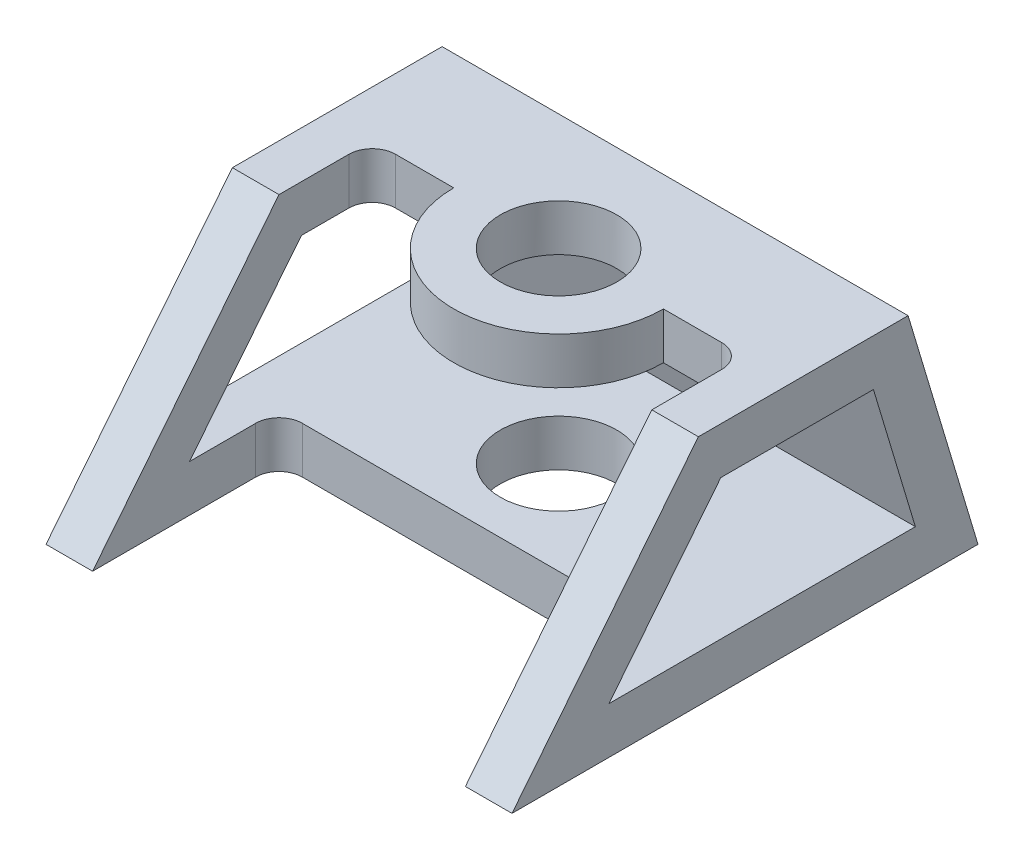
ISO-10303-21;
HEADER;
FILE_DESCRIPTION(('STEP AP214'),'2;1');
FILE_NAME('part.step','',(''),(''),'','','');
FILE_SCHEMA(('AUTOMOTIVE_DESIGN { 1 0 10303 214 1 1 1 1 }'));
ENDSEC;
DATA;
#1=APPLICATION_CONTEXT('core data for automotive mechanical design processes');
#2=APPLICATION_PROTOCOL_DEFINITION('international standard','automotive_design',2000,#1);
#3=PRODUCT_CONTEXT('',#1,'mechanical');
#4=PRODUCT('Part','Part','',(#3));
#5=PRODUCT_RELATED_PRODUCT_CATEGORY('part','',(#4));
#6=PRODUCT_DEFINITION_FORMATION('','',#4);
#7=PRODUCT_DEFINITION_CONTEXT('part definition',#1,'design');
#8=PRODUCT_DEFINITION('design','',#6,#7);
#9=PRODUCT_DEFINITION_SHAPE('','',#8);
#10=(LENGTH_UNIT() NAMED_UNIT(*) SI_UNIT(.MILLI.,.METRE.));
#11=(NAMED_UNIT(*) PLANE_ANGLE_UNIT() SI_UNIT($,.RADIAN.));
#12=(NAMED_UNIT(*) SI_UNIT($,.STERADIAN.) SOLID_ANGLE_UNIT());
#13=UNCERTAINTY_MEASURE_WITH_UNIT(LENGTH_MEASURE(1.E-05),#10,'distance_accuracy_value','');
#14=(GEOMETRIC_REPRESENTATION_CONTEXT(3) GLOBAL_UNCERTAINTY_ASSIGNED_CONTEXT((#13)) GLOBAL_UNIT_ASSIGNED_CONTEXT((#10,
#11,#12)) REPRESENTATION_CONTEXT('',''));
#15=CARTESIAN_POINT('',(0.,0.,0.));
#16=DIRECTION('',(0.,0.,1.));
#17=DIRECTION('',(1.,0.,0.));
#18=AXIS2_PLACEMENT_3D('',#15,#16,#17);
#19=CARTESIAN_POINT('',(-80.,-0.00100000000001488,-120.));
#20=DIRECTION('',(0.,0.,-1.));
#21=DIRECTION('',(0.,1.,0.));
#22=AXIS2_PLACEMENT_3D('',#19,#20,#21);
#23=PLANE('',#22);
#24=DIRECTION('',(-1.,0.,0.));
#25=VECTOR('',#24,1.);
#26=CARTESIAN_POINT('',(-80.,80.,-120.));
#27=LINE('',#26,#25);
#28=CARTESIAN_POINT('',(-45.,80.,-120.));
#29=VERTEX_POINT('',#28);
#30=CARTESIAN_POINT('',(-70.,80.,-120.));
#31=VERTEX_POINT('',#30);
#32=EDGE_CURVE('E339',#29,#31,#27,.T.);
#33=ORIENTED_EDGE('',*,*,#32,.F.);
#34=DIRECTION('',(0.,1.,0.));
#35=VECTOR('',#34,1.);
#36=CARTESIAN_POINT('',(-45.,-47.2792206135785,-120.));
#37=LINE('',#36,#35);
#38=CARTESIAN_POINT('',(-45.,100.,-120.));
#39=VERTEX_POINT('',#38);
#40=EDGE_CURVE('E11',#29,#39,#37,.T.);
#41=ORIENTED_EDGE('',*,*,#40,.T.);
#42=DIRECTION('',(-1.,0.,0.));
#43=VECTOR('',#42,1.);
#44=CARTESIAN_POINT('',(-80.,100.,-120.));
#45=LINE('',#44,#43);
#46=CARTESIAN_POINT('',(-70.,100.,-120.));
#47=VERTEX_POINT('',#46);
#48=EDGE_CURVE('E205',#39,#47,#45,.T.);
#49=ORIENTED_EDGE('',*,*,#48,.T.);
#50=DIRECTION('',(0.,1.,0.));
#51=VECTOR('',#50,1.);
#52=CARTESIAN_POINT('',(-70.,80.,-120.));
#53=LINE('',#52,#51);
#54=EDGE_CURVE('E310',#47,#31,#53,.F.);
#55=ORIENTED_EDGE('',*,*,#54,.T.);
#56=EDGE_LOOP('',(#33,#41,#49,#55));
#57=FACE_BOUND('',#56,.T.);
#58=ADVANCED_FACE('F39',(#57),#23,.F.);
#59=CARTESIAN_POINT('',(100.,100.,-80.));
#60=DIRECTION('',(0.,-0.624695047554424,-0.78086880944303));
#61=DIRECTION('',(0.,0.78086880944303,-0.624695047554424));
#62=AXIS2_PLACEMENT_3D('',#59,#60,#61);
#63=PLANE('',#62);
#64=DIRECTION('',(-1.,0.,0.));
#65=VECTOR('',#64,1.);
#66=CARTESIAN_POINT('',(100.,0.,0.));
#67=LINE('',#66,#65);
#68=CARTESIAN_POINT('',(-80.,0.,0.));
#69=VERTEX_POINT('',#68);
#70=CARTESIAN_POINT('',(-100.,0.,0.));
#71=VERTEX_POINT('',#70);
#72=EDGE_CURVE('E273',#69,#71,#67,.T.);
#73=ORIENTED_EDGE('',*,*,#72,.F.);
#74=DIRECTION('',(0.,0.78086880944303,-0.624695047554424));
#75=VECTOR('',#74,1.);
#76=CARTESIAN_POINT('',(-80.,100.,-80.));
#77=LINE('',#76,#75);
#78=CARTESIAN_POINT('',(-80.,100.,-80.));
#79=VERTEX_POINT('',#78);
#80=EDGE_CURVE('E227',#69,#79,#77,.T.);
#81=ORIENTED_EDGE('',*,*,#80,.T.);
#82=DIRECTION('',(-1.,0.,0.));
#83=VECTOR('',#82,1.);
#84=CARTESIAN_POINT('',(100.,100.,-80.));
#85=LINE('',#84,#83);
#86=CARTESIAN_POINT('',(-100.,100.,-80.));
#87=VERTEX_POINT('',#86);
#88=EDGE_CURVE('E290',#79,#87,#85,.T.);
#89=ORIENTED_EDGE('',*,*,#88,.T.);
#90=DIRECTION('',(0.,-0.78086880944303,0.624695047554424));
#91=VECTOR('',#90,1.);
#92=CARTESIAN_POINT('',(-100.,100.,-80.));
#93=LINE('',#92,#91);
#94=EDGE_CURVE('E268',#87,#71,#93,.T.);
#95=ORIENTED_EDGE('',*,*,#94,.T.);
#96=EDGE_LOOP('',(#73,#81,#89,#95));
#97=FACE_BOUND('',#96,.T.);
#98=ADVANCED_FACE('F409',(#97),#63,.F.);
#99=CARTESIAN_POINT('',(100.,80.,-89.6124969497314));
#100=DIRECTION('',(0.,-0.624695047554424,-0.78086880944303));
#101=DIRECTION('',(0.,0.78086880944303,-0.624695047554424));
#102=AXIS2_PLACEMENT_3D('',#99,#100,#101);
#103=PLANE('',#102);
#104=DIRECTION('',(0.,0.78086880944303,-0.624695047554424));
#105=VECTOR('',#104,1.);
#106=CARTESIAN_POINT('',(-80.,80.,-89.6124969497314));
#107=LINE('',#106,#105);
#108=CARTESIAN_POINT('',(-80.,20.,-41.6124969497314));
#109=VERTEX_POINT('',#108);
#110=CARTESIAN_POINT('',(-80.,80.,-89.6124969497314));
#111=VERTEX_POINT('',#110);
#112=EDGE_CURVE('E224',#109,#111,#107,.T.);
#113=ORIENTED_EDGE('',*,*,#112,.F.);
#114=DIRECTION('',(-1.,0.,0.));
#115=VECTOR('',#114,1.);
#116=CARTESIAN_POINT('',(100.,20.,-41.6124969497314));
#117=LINE('',#116,#115);
#118=CARTESIAN_POINT('',(-100.,20.,-41.6124969497314));
#119=VERTEX_POINT('',#118);
#120=EDGE_CURVE('E251',#109,#119,#117,.T.);
#121=ORIENTED_EDGE('',*,*,#120,.T.);
#122=DIRECTION('',(0.,-0.78086880944303,0.624695047554424));
#123=VECTOR('',#122,1.);
#124=CARTESIAN_POINT('',(-100.,80.,-89.6124969497314));
#125=LINE('',#124,#123);
#126=CARTESIAN_POINT('',(-100.,80.,-89.6124969497314));
#127=VERTEX_POINT('',#126);
#128=EDGE_CURVE('E248',#127,#119,#125,.T.);
#129=ORIENTED_EDGE('',*,*,#128,.F.);
#130=DIRECTION('',(-1.,0.,0.));
#131=VECTOR('',#130,1.);
#132=CARTESIAN_POINT('',(100.,80.,-89.6124969497314));
#133=LINE('',#132,#131);
#134=EDGE_CURVE('E260',#111,#127,#133,.T.);
#135=ORIENTED_EDGE('',*,*,#134,.F.);
#136=EDGE_LOOP('',(#113,#121,#129,#135));
#137=FACE_BOUND('',#136,.T.);
#138=ADVANCED_FACE('F391',(#137),#103,.T.);
#139=CARTESIAN_POINT('',(100.,0.,0.));
#140=DIRECTION('',(1.,0.,0.));
#141=DIRECTION('',(0.,0.,-1.));
#142=AXIS2_PLACEMENT_3D('',#139,#140,#141);
#143=PLANE('',#142);
#144=DIRECTION('',(0.,0.,-1.));
#145=VECTOR('',#144,1.);
#146=CARTESIAN_POINT('',(100.,0.,0.));
#147=LINE('',#146,#145);
#148=CARTESIAN_POINT('',(100.,0.,0.));
#149=VERTEX_POINT('',#148);
#150=CARTESIAN_POINT('',(100.,0.,-200.));
#151=VERTEX_POINT('',#150);
#152=EDGE_CURVE('E262',#149,#151,#147,.T.);
#153=ORIENTED_EDGE('',*,*,#152,.T.);
#154=DIRECTION('',(0.,0.957826285221151,0.287347885566345));
#155=VECTOR('',#154,1.);
#156=CARTESIAN_POINT('',(100.,0.,-200.));
#157=LINE('',#156,#155);
#158=CARTESIAN_POINT('',(100.,100.,-170.));
#159=VERTEX_POINT('',#158);
#160=EDGE_CURVE('E270',#151,#159,#157,.T.);
#161=ORIENTED_EDGE('',*,*,#160,.T.);
#162=DIRECTION('',(0.,0.,1.));
#163=VECTOR('',#162,1.);
#164=CARTESIAN_POINT('',(100.,100.,-170.));
#165=LINE('',#164,#163);
#166=CARTESIAN_POINT('',(100.,100.,-80.));
#167=VERTEX_POINT('',#166);
#168=EDGE_CURVE('E269',#159,#167,#165,.T.);
#169=ORIENTED_EDGE('',*,*,#168,.T.);
#170=DIRECTION('',(0.,-0.78086880944303,0.624695047554424));
#171=VECTOR('',#170,1.);
#172=CARTESIAN_POINT('',(100.,100.,-80.));
#173=LINE('',#172,#171);
#174=EDGE_CURVE('E275',#167,#149,#173,.T.);
#175=ORIENTED_EDGE('',*,*,#174,.T.);
#176=EDGE_LOOP('',(#153,#161,#169,#175));
#177=FACE_BOUND('',#176,.T.);
#178=DIRECTION('',(0.,0.,1.));
#179=VECTOR('',#178,1.);
#180=CARTESIAN_POINT('',(100.,80.,-155.119386982179));
#181=LINE('',#180,#179);
#182=CARTESIAN_POINT('',(100.,80.,-155.119386982179));
#183=VERTEX_POINT('',#182);
#184=CARTESIAN_POINT('',(100.,80.,-89.6124969497314));
#185=VERTEX_POINT('',#184);
#186=EDGE_CURVE('E235',#183,#185,#181,.T.);
#187=ORIENTED_EDGE('',*,*,#186,.F.);
#188=DIRECTION('',(0.,0.957826285221152,0.287347885566345));
#189=VECTOR('',#188,1.);
#190=CARTESIAN_POINT('',(100.,20.,-173.119386982179));
#191=LINE('',#190,#189);
#192=CARTESIAN_POINT('',(100.,20.,-173.119386982179));
#193=VERTEX_POINT('',#192);
#194=EDGE_CURVE('E228',#193,#183,#191,.T.);
#195=ORIENTED_EDGE('',*,*,#194,.F.);
#196=DIRECTION('',(0.,0.,-1.));
#197=VECTOR('',#196,1.);
#198=CARTESIAN_POINT('',(100.,20.,-41.6124969497314));
#199=LINE('',#198,#197);
#200=CARTESIAN_POINT('',(100.,20.,-41.6124969497314));
#201=VERTEX_POINT('',#200);
#202=EDGE_CURVE('E236',#201,#193,#199,.T.);
#203=ORIENTED_EDGE('',*,*,#202,.F.);
#204=DIRECTION('',(0.,-0.78086880944303,0.624695047554424));
#205=VECTOR('',#204,1.);
#206=CARTESIAN_POINT('',(100.,80.,-89.6124969497314));
#207=LINE('',#206,#205);
#208=EDGE_CURVE('E232',#185,#201,#207,.T.);
#209=ORIENTED_EDGE('',*,*,#208,.F.);
#210=EDGE_LOOP('',(#187,#195,#203,#209));
#211=FACE_BOUND('',#210,.T.);
#212=ADVANCED_FACE('F435',(#177,#211),#143,.T.);
#213=CARTESIAN_POINT('',(-100.,0.,0.));
#214=DIRECTION('',(1.,0.,0.));
#215=DIRECTION('',(0.,0.,-1.));
#216=AXIS2_PLACEMENT_3D('',#213,#214,#215);
#217=PLANE('',#216);
#218=DIRECTION('',(0.,0.,-1.));
#219=VECTOR('',#218,1.);
#220=CARTESIAN_POINT('',(-100.,0.,0.));
#221=LINE('',#220,#219);
#222=CARTESIAN_POINT('',(-100.,0.,-200.));
#223=VERTEX_POINT('',#222);
#224=EDGE_CURVE('E263',#71,#223,#221,.T.);
#225=ORIENTED_EDGE('',*,*,#224,.F.);
#226=ORIENTED_EDGE('',*,*,#94,.F.);
#227=DIRECTION('',(0.,0.,1.));
#228=VECTOR('',#227,1.);
#229=CARTESIAN_POINT('',(-100.,100.,-170.));
#230=LINE('',#229,#228);
#231=CARTESIAN_POINT('',(-100.,100.,-170.));
#232=VERTEX_POINT('',#231);
#233=EDGE_CURVE('E276',#232,#87,#230,.T.);
#234=ORIENTED_EDGE('',*,*,#233,.F.);
#235=DIRECTION('',(0.,0.957826285221151,0.287347885566345));
#236=VECTOR('',#235,1.);
#237=CARTESIAN_POINT('',(-100.,0.,-200.));
#238=LINE('',#237,#236);
#239=EDGE_CURVE('E280',#223,#232,#238,.T.);
#240=ORIENTED_EDGE('',*,*,#239,.F.);
#241=EDGE_LOOP('',(#225,#226,#234,#240));
#242=FACE_BOUND('',#241,.T.);
#243=DIRECTION('',(0.,0.957826285221152,0.287347885566345));
#244=VECTOR('',#243,1.);
#245=CARTESIAN_POINT('',(-100.,20.,-173.119386982179));
#246=LINE('',#245,#244);
#247=CARTESIAN_POINT('',(-100.,20.,-173.119386982179));
#248=VERTEX_POINT('',#247);
#249=CARTESIAN_POINT('',(-100.,80.,-155.119386982179));
#250=VERTEX_POINT('',#249);
#251=EDGE_CURVE('E226',#248,#250,#246,.T.);
#252=ORIENTED_EDGE('',*,*,#251,.T.);
#253=DIRECTION('',(0.,0.,1.));
#254=VECTOR('',#253,1.);
#255=CARTESIAN_POINT('',(-100.,80.,-155.119386982179));
#256=LINE('',#255,#254);
#257=EDGE_CURVE('E245',#250,#127,#256,.T.);
#258=ORIENTED_EDGE('',*,*,#257,.T.);
#259=ORIENTED_EDGE('',*,*,#128,.T.);
#260=DIRECTION('',(0.,0.,-1.));
#261=VECTOR('',#260,1.);
#262=CARTESIAN_POINT('',(-100.,20.,-41.6124969497314));
#263=LINE('',#262,#261);
#264=EDGE_CURVE('E231',#119,#248,#263,.T.);
#265=ORIENTED_EDGE('',*,*,#264,.T.);
#266=EDGE_LOOP('',(#252,#258,#259,#265));
#267=FACE_BOUND('',#266,.T.);
#268=ADVANCED_FACE('F437',(#242,#267),#217,.F.);
#269=CARTESIAN_POINT('',(100.,0.,0.));
#270=DIRECTION('',(0.,1.,0.));
#271=DIRECTION('',(0.,0.,1.));
#272=AXIS2_PLACEMENT_3D('',#269,#270,#271);
#273=PLANE('',#272);
#274=CARTESIAN_POINT('',(0.,0.,-120.));
#275=DIRECTION('',(0.,1.,0.));
#276=DIRECTION('',(0.,0.,1.));
#277=AXIS2_PLACEMENT_3D('',#274,#275,#276);
#278=CIRCLE('',#277,25.);
#279=CARTESIAN_POINT('',(0.,0.,-95.));
#280=VERTEX_POINT('',#279);
#281=EDGE_CURVE('E369',#280,#280,#278,.T.);
#282=ORIENTED_EDGE('',*,*,#281,.T.);
#283=EDGE_LOOP('',(#282));
#284=FACE_BOUND('',#283,.T.);
#285=DIRECTION('',(1.,0.,0.));
#286=VECTOR('',#285,1.);
#287=CARTESIAN_POINT('',(-80.,0.,-80.));
#288=LINE('',#287,#286);
#289=CARTESIAN_POINT('',(-70.,0.,-80.));
#290=VERTEX_POINT('',#289);
#291=CARTESIAN_POINT('',(70.,0.,-80.));
#292=VERTEX_POINT('',#291);
#293=EDGE_CURVE('E356',#290,#292,#288,.T.);
#294=ORIENTED_EDGE('',*,*,#293,.F.);
#295=CARTESIAN_POINT('',(-70.,0.,-70.));
#296=DIRECTION('',(0.,1.,0.));
#297=DIRECTION('',(0.,0.,1.));
#298=AXIS2_PLACEMENT_3D('',#295,#296,#297);
#299=CIRCLE('',#298,10.);
#300=CARTESIAN_POINT('',(-80.,0.,-70.));
#301=VERTEX_POINT('',#300);
#302=EDGE_CURVE('E320',#290,#301,#299,.T.);
#303=ORIENTED_EDGE('',*,*,#302,.T.);
#304=DIRECTION('',(0.,0.,-1.));
#305=VECTOR('',#304,1.);
#306=CARTESIAN_POINT('',(-80.,0.,0.));
#307=LINE('',#306,#305);
#308=EDGE_CURVE('E353',#69,#301,#307,.T.);
#309=ORIENTED_EDGE('',*,*,#308,.F.);
#310=ORIENTED_EDGE('',*,*,#72,.T.);
#311=ORIENTED_EDGE('',*,*,#224,.T.);
#312=DIRECTION('',(-1.,0.,0.));
#313=VECTOR('',#312,1.);
#314=CARTESIAN_POINT('',(100.,0.,-200.));
#315=LINE('',#314,#313);
#316=EDGE_CURVE('E294',#151,#223,#315,.T.);
#317=ORIENTED_EDGE('',*,*,#316,.F.);
#318=ORIENTED_EDGE('',*,*,#152,.F.);
#319=CARTESIAN_POINT('',(80.,0.,0.));
#320=VERTEX_POINT('',#319);
#321=EDGE_CURVE('E281',#149,#320,#67,.T.);
#322=ORIENTED_EDGE('',*,*,#321,.T.);
#323=DIRECTION('',(0.,0.,1.));
#324=VECTOR('',#323,1.);
#325=CARTESIAN_POINT('',(80.,0.,0.));
#326=LINE('',#325,#324);
#327=CARTESIAN_POINT('',(80.,0.,-70.));
#328=VERTEX_POINT('',#327);
#329=EDGE_CURVE('E363',#328,#320,#326,.T.);
#330=ORIENTED_EDGE('',*,*,#329,.F.);
#331=CARTESIAN_POINT('',(70.,0.,-70.));
#332=DIRECTION('',(0.,1.,0.));
#333=DIRECTION('',(0.,0.,1.));
#334=AXIS2_PLACEMENT_3D('',#331,#332,#333);
#335=CIRCLE('',#334,10.);
#336=EDGE_CURVE('E324',#328,#292,#335,.T.);
#337=ORIENTED_EDGE('',*,*,#336,.T.);
#338=EDGE_LOOP('',(#294,#303,#309,#310,#311,#317,#318,#322,#330,#337));
#339=FACE_BOUND('',#338,.T.);
#340=ADVANCED_FACE('F415',(#284,#339),#273,.F.);
#341=CARTESIAN_POINT('',(100.,0.,-200.));
#342=DIRECTION('',(0.,-0.287347885566345,0.957826285221152));
#343=DIRECTION('',(0.,-0.957826285221152,-0.287347885566345));
#344=AXIS2_PLACEMENT_3D('',#341,#342,#343);
#345=PLANE('',#344);
#346=ORIENTED_EDGE('',*,*,#239,.T.);
#347=DIRECTION('',(-1.,0.,0.));
#348=VECTOR('',#347,1.);
#349=CARTESIAN_POINT('',(100.,100.,-170.));
#350=LINE('',#349,#348);
#351=EDGE_CURVE('E292',#159,#232,#350,.T.);
#352=ORIENTED_EDGE('',*,*,#351,.F.);
#353=ORIENTED_EDGE('',*,*,#160,.F.);
#354=ORIENTED_EDGE('',*,*,#316,.T.);
#355=EDGE_LOOP('',(#346,#352,#353,#354));
#356=FACE_BOUND('',#355,.T.);
#357=ADVANCED_FACE('F436',(#356),#345,.F.);
#358=CARTESIAN_POINT('',(100.,100.,-170.));
#359=DIRECTION('',(0.,-1.,0.));
#360=DIRECTION('',(0.,0.,-1.));
#361=AXIS2_PLACEMENT_3D('',#358,#359,#360);
#362=PLANE('',#361);
#363=CARTESIAN_POINT('',(0.,100.,-120.));
#364=DIRECTION('',(0.,1.,0.));
#365=DIRECTION('',(0.,0.,1.));
#366=AXIS2_PLACEMENT_3D('',#363,#364,#365);
#367=CIRCLE('',#366,25.);
#368=CARTESIAN_POINT('',(0.,100.,-95.));
#369=VERTEX_POINT('',#368);
#370=EDGE_CURVE('E368',#369,#369,#367,.T.);
#371=ORIENTED_EDGE('',*,*,#370,.F.);
#372=EDGE_LOOP('',(#371));
#373=FACE_BOUND('',#372,.T.);
#374=ORIENTED_EDGE('',*,*,#48,.F.);
#375=CARTESIAN_POINT('',(0.,100.,-120.));
#376=DIRECTION('',(0.,1.,0.));
#377=DIRECTION('',(0.,0.,1.));
#378=AXIS2_PLACEMENT_3D('',#375,#376,#377);
#379=CIRCLE('',#378,45.);
#380=CARTESIAN_POINT('',(45.,100.,-120.));
#381=VERTEX_POINT('',#380);
#382=EDGE_CURVE('E186',#39,#381,#379,.T.);
#383=ORIENTED_EDGE('',*,*,#382,.T.);
#384=CARTESIAN_POINT('',(70.,100.,-120.));
#385=VERTEX_POINT('',#384);
#386=EDGE_CURVE('E199',#385,#381,#45,.T.);
#387=ORIENTED_EDGE('',*,*,#386,.F.);
#388=CARTESIAN_POINT('',(70.,100.,-110.));
#389=DIRECTION('',(0.,-1.,0.));
#390=DIRECTION('',(0.,0.,-1.));
#391=AXIS2_PLACEMENT_3D('',#388,#389,#390);
#392=CIRCLE('',#391,10.);
#393=CARTESIAN_POINT('',(80.,100.,-110.));
#394=VERTEX_POINT('',#393);
#395=EDGE_CURVE('E330',#385,#394,#392,.T.);
#396=ORIENTED_EDGE('',*,*,#395,.T.);
#397=DIRECTION('',(0.,0.,-1.));
#398=VECTOR('',#397,1.);
#399=CARTESIAN_POINT('',(80.,100.,-120.));
#400=LINE('',#399,#398);
#401=CARTESIAN_POINT('',(80.,100.,-80.));
#402=VERTEX_POINT('',#401);
#403=EDGE_CURVE('E212',#402,#394,#400,.T.);
#404=ORIENTED_EDGE('',*,*,#403,.F.);
#405=EDGE_CURVE('E286',#167,#402,#85,.T.);
#406=ORIENTED_EDGE('',*,*,#405,.F.);
#407=ORIENTED_EDGE('',*,*,#168,.F.);
#408=ORIENTED_EDGE('',*,*,#351,.T.);
#409=ORIENTED_EDGE('',*,*,#233,.T.);
#410=ORIENTED_EDGE('',*,*,#88,.F.);
#411=DIRECTION('',(0.,0.,1.));
#412=VECTOR('',#411,1.);
#413=CARTESIAN_POINT('',(-80.,100.,-120.));
#414=LINE('',#413,#412);
#415=CARTESIAN_POINT('',(-80.,100.,-110.));
#416=VERTEX_POINT('',#415);
#417=EDGE_CURVE('E341',#416,#79,#414,.T.);
#418=ORIENTED_EDGE('',*,*,#417,.F.);
#419=CARTESIAN_POINT('',(-70.,100.,-110.));
#420=DIRECTION('',(0.,-1.,0.));
#421=DIRECTION('',(0.,0.,-1.));
#422=AXIS2_PLACEMENT_3D('',#419,#420,#421);
#423=CIRCLE('',#422,10.);
#424=EDGE_CURVE('E317',#416,#47,#423,.T.);
#425=ORIENTED_EDGE('',*,*,#424,.T.);
#426=EDGE_LOOP('',(#374,#383,#387,#396,#404,#406,#407,#408,#409,#410,#418,#425));
#427=FACE_BOUND('',#426,.T.);
#428=ADVANCED_FACE('F200',(#373,#427),#362,.F.);
#429=DIRECTION('',(0.,-0.78086880944303,0.624695047554424));
#430=VECTOR('',#429,1.);
#431=CARTESIAN_POINT('',(80.,100.,-80.));
#432=LINE('',#431,#430);
#433=EDGE_CURVE('E219',#402,#320,#432,.T.);
#434=ORIENTED_EDGE('',*,*,#433,.T.);
#435=ORIENTED_EDGE('',*,*,#321,.F.);
#436=ORIENTED_EDGE('',*,*,#174,.F.);
#437=ORIENTED_EDGE('',*,*,#405,.T.);
#438=EDGE_LOOP('',(#434,#435,#436,#437));
#439=FACE_BOUND('',#438,.T.);
#440=ADVANCED_FACE('F430',(#439),#63,.F.);
#441=CARTESIAN_POINT('',(100.,20.,-173.119386982179));
#442=DIRECTION('',(0.,-0.287347885566345,0.957826285221151));
#443=DIRECTION('',(0.,-0.957826285221152,-0.287347885566345));
#444=AXIS2_PLACEMENT_3D('',#441,#442,#443);
#445=PLANE('',#444);
#446=ORIENTED_EDGE('',*,*,#251,.F.);
#447=DIRECTION('',(-1.,0.,0.));
#448=VECTOR('',#447,1.);
#449=CARTESIAN_POINT('',(100.,20.,-173.119386982179));
#450=LINE('',#449,#448);
#451=EDGE_CURVE('E238',#193,#248,#450,.T.);
#452=ORIENTED_EDGE('',*,*,#451,.F.);
#453=ORIENTED_EDGE('',*,*,#194,.T.);
#454=DIRECTION('',(-1.,0.,0.));
#455=VECTOR('',#454,1.);
#456=CARTESIAN_POINT('',(100.,80.,-155.119386982179));
#457=LINE('',#456,#455);
#458=EDGE_CURVE('E261',#183,#250,#457,.T.);
#459=ORIENTED_EDGE('',*,*,#458,.T.);
#460=EDGE_LOOP('',(#446,#452,#453,#459));
#461=FACE_BOUND('',#460,.T.);
#462=ADVANCED_FACE('F441',(#461),#445,.T.);
#463=CARTESIAN_POINT('',(100.,80.,-155.119386982179));
#464=DIRECTION('',(0.,-1.,0.));
#465=DIRECTION('',(0.,0.,-1.));
#466=AXIS2_PLACEMENT_3D('',#463,#464,#465);
#467=PLANE('',#466);
#468=CARTESIAN_POINT('',(0.,80.,-120.));
#469=DIRECTION('',(0.,-1.,0.));
#470=DIRECTION('',(0.,0.,-1.));
#471=AXIS2_PLACEMENT_3D('',#468,#469,#470);
#472=CIRCLE('',#471,25.);
#473=CARTESIAN_POINT('',(0.,80.,-145.));
#474=VERTEX_POINT('',#473);
#475=EDGE_CURVE('E201',#474,#474,#472,.T.);
#476=ORIENTED_EDGE('',*,*,#475,.F.);
#477=EDGE_LOOP('',(#476));
#478=FACE_BOUND('',#477,.T.);
#479=ORIENTED_EDGE('',*,*,#257,.F.);
#480=ORIENTED_EDGE('',*,*,#458,.F.);
#481=ORIENTED_EDGE('',*,*,#186,.T.);
#482=CARTESIAN_POINT('',(80.,80.,-89.6124969497314));
#483=VERTEX_POINT('',#482);
#484=EDGE_CURVE('E256',#185,#483,#133,.T.);
#485=ORIENTED_EDGE('',*,*,#484,.T.);
#486=DIRECTION('',(0.,0.,-1.));
#487=VECTOR('',#486,1.);
#488=CARTESIAN_POINT('',(80.,80.,-120.));
#489=LINE('',#488,#487);
#490=CARTESIAN_POINT('',(80.,80.,-110.));
#491=VERTEX_POINT('',#490);
#492=EDGE_CURVE('E207',#483,#491,#489,.T.);
#493=ORIENTED_EDGE('',*,*,#492,.T.);
#494=CARTESIAN_POINT('',(70.,80.,-110.));
#495=DIRECTION('',(0.,-1.,0.));
#496=DIRECTION('',(0.,0.,-1.));
#497=AXIS2_PLACEMENT_3D('',#494,#495,#496);
#498=CIRCLE('',#497,10.);
#499=CARTESIAN_POINT('',(70.,80.,-120.));
#500=VERTEX_POINT('',#499);
#501=EDGE_CURVE('E194',#491,#500,#498,.F.);
#502=ORIENTED_EDGE('',*,*,#501,.T.);
#503=CARTESIAN_POINT('',(45.,80.,-120.));
#504=VERTEX_POINT('',#503);
#505=EDGE_CURVE('E334',#500,#504,#27,.T.);
#506=ORIENTED_EDGE('',*,*,#505,.T.);
#507=CARTESIAN_POINT('',(0.,80.,-120.));
#508=DIRECTION('',(0.,-1.,0.));
#509=DIRECTION('',(0.,0.,-1.));
#510=AXIS2_PLACEMENT_3D('',#507,#508,#509);
#511=CIRCLE('',#510,45.);
#512=EDGE_CURVE('E54',#29,#504,#511,.F.);
#513=ORIENTED_EDGE('',*,*,#512,.F.);
#514=ORIENTED_EDGE('',*,*,#32,.T.);
#515=CARTESIAN_POINT('',(-70.,80.,-110.));
#516=DIRECTION('',(0.,-1.,0.));
#517=DIRECTION('',(0.,0.,-1.));
#518=AXIS2_PLACEMENT_3D('',#515,#516,#517);
#519=CIRCLE('',#518,10.);
#520=CARTESIAN_POINT('',(-80.,80.,-110.));
#521=VERTEX_POINT('',#520);
#522=EDGE_CURVE('E321',#31,#521,#519,.F.);
#523=ORIENTED_EDGE('',*,*,#522,.T.);
#524=DIRECTION('',(0.,0.,1.));
#525=VECTOR('',#524,1.);
#526=CARTESIAN_POINT('',(-80.,80.,-120.));
#527=LINE('',#526,#525);
#528=EDGE_CURVE('E337',#521,#111,#527,.T.);
#529=ORIENTED_EDGE('',*,*,#528,.T.);
#530=ORIENTED_EDGE('',*,*,#134,.T.);
#531=EDGE_LOOP('',(#479,#480,#481,#485,#493,#502,#506,#513,#514,#523,#529,#530));
#532=FACE_BOUND('',#531,.T.);
#533=ADVANCED_FACE('F335',(#478,#532),#467,.T.);
#534=DIRECTION('',(0.,-0.78086880944303,0.624695047554424));
#535=VECTOR('',#534,1.);
#536=CARTESIAN_POINT('',(80.,80.,-89.6124969497314));
#537=LINE('',#536,#535);
#538=CARTESIAN_POINT('',(80.,20.,-41.6124969497314));
#539=VERTEX_POINT('',#538);
#540=EDGE_CURVE('E215',#483,#539,#537,.T.);
#541=ORIENTED_EDGE('',*,*,#540,.F.);
#542=ORIENTED_EDGE('',*,*,#484,.F.);
#543=ORIENTED_EDGE('',*,*,#208,.T.);
#544=EDGE_CURVE('E255',#201,#539,#117,.T.);
#545=ORIENTED_EDGE('',*,*,#544,.T.);
#546=EDGE_LOOP('',(#541,#542,#543,#545));
#547=FACE_BOUND('',#546,.T.);
#548=ADVANCED_FACE('F382',(#547),#103,.T.);
#549=CARTESIAN_POINT('',(100.,20.,-41.6124969497314));
#550=DIRECTION('',(0.,1.,0.));
#551=DIRECTION('',(0.,0.,1.));
#552=AXIS2_PLACEMENT_3D('',#549,#550,#551);
#553=PLANE('',#552);
#554=CARTESIAN_POINT('',(0.,20.,-120.));
#555=DIRECTION('',(0.,1.,0.));
#556=DIRECTION('',(0.,0.,1.));
#557=AXIS2_PLACEMENT_3D('',#554,#555,#556);
#558=CIRCLE('',#557,25.);
#559=CARTESIAN_POINT('',(0.,20.,-95.));
#560=VERTEX_POINT('',#559);
#561=EDGE_CURVE('E43',#560,#560,#558,.T.);
#562=ORIENTED_EDGE('',*,*,#561,.F.);
#563=EDGE_LOOP('',(#562));
#564=FACE_BOUND('',#563,.T.);
#565=DIRECTION('',(0.,0.,1.));
#566=VECTOR('',#565,1.);
#567=CARTESIAN_POINT('',(-80.,20.,0.));
#568=LINE('',#567,#566);
#569=CARTESIAN_POINT('',(-80.,20.,-70.));
#570=VERTEX_POINT('',#569);
#571=EDGE_CURVE('E355',#570,#109,#568,.T.);
#572=ORIENTED_EDGE('',*,*,#571,.F.);
#573=CARTESIAN_POINT('',(-70.,20.,-70.));
#574=DIRECTION('',(0.,1.,0.));
#575=DIRECTION('',(0.,0.,1.));
#576=AXIS2_PLACEMENT_3D('',#573,#574,#575);
#577=CIRCLE('',#576,10.);
#578=CARTESIAN_POINT('',(-70.,20.,-80.));
#579=VERTEX_POINT('',#578);
#580=EDGE_CURVE('E312',#570,#579,#577,.F.);
#581=ORIENTED_EDGE('',*,*,#580,.T.);
#582=DIRECTION('',(-1.,0.,0.));
#583=VECTOR('',#582,1.);
#584=CARTESIAN_POINT('',(-80.,20.,-80.));
#585=LINE('',#584,#583);
#586=CARTESIAN_POINT('',(70.,20.,-80.));
#587=VERTEX_POINT('',#586);
#588=EDGE_CURVE('E346',#587,#579,#585,.T.);
#589=ORIENTED_EDGE('',*,*,#588,.F.);
#590=CARTESIAN_POINT('',(70.,20.,-70.));
#591=DIRECTION('',(0.,1.,0.));
#592=DIRECTION('',(0.,0.,1.));
#593=AXIS2_PLACEMENT_3D('',#590,#591,#592);
#594=CIRCLE('',#593,10.);
#595=CARTESIAN_POINT('',(80.,20.,-70.));
#596=VERTEX_POINT('',#595);
#597=EDGE_CURVE('E323',#587,#596,#594,.F.);
#598=ORIENTED_EDGE('',*,*,#597,.T.);
#599=DIRECTION('',(0.,0.,-1.));
#600=VECTOR('',#599,1.);
#601=CARTESIAN_POINT('',(80.,20.,0.));
#602=LINE('',#601,#600);
#603=EDGE_CURVE('E352',#539,#596,#602,.T.);
#604=ORIENTED_EDGE('',*,*,#603,.F.);
#605=ORIENTED_EDGE('',*,*,#544,.F.);
#606=ORIENTED_EDGE('',*,*,#202,.T.);
#607=ORIENTED_EDGE('',*,*,#451,.T.);
#608=ORIENTED_EDGE('',*,*,#264,.F.);
#609=ORIENTED_EDGE('',*,*,#120,.F.);
#610=EDGE_LOOP('',(#572,#581,#589,#598,#604,#605,#606,#607,#608,#609));
#611=FACE_BOUND('',#610,.T.);
#612=ADVANCED_FACE('F377',(#564,#611),#553,.T.);
#613=CARTESIAN_POINT('',(-80.,80.,-150.));
#614=DIRECTION('',(-1.,0.,0.));
#615=DIRECTION('',(0.,-1.,0.));
#616=AXIS2_PLACEMENT_3D('',#613,#614,#615);
#617=PLANE('',#616);
#618=ORIENTED_EDGE('',*,*,#308,.T.);
#619=DIRECTION('',(0.,1.,0.));
#620=VECTOR('',#619,1.);
#621=CARTESIAN_POINT('',(-80.,20.,-70.));
#622=LINE('',#621,#620);
#623=EDGE_CURVE('E298',#301,#570,#622,.T.);
#624=ORIENTED_EDGE('',*,*,#623,.T.);
#625=ORIENTED_EDGE('',*,*,#571,.T.);
#626=ORIENTED_EDGE('',*,*,#112,.T.);
#627=ORIENTED_EDGE('',*,*,#528,.F.);
#628=DIRECTION('',(0.,1.,0.));
#629=VECTOR('',#628,1.);
#630=CARTESIAN_POINT('',(-80.,100.,-110.));
#631=LINE('',#630,#629);
#632=EDGE_CURVE('E299',#521,#416,#631,.T.);
#633=ORIENTED_EDGE('',*,*,#632,.T.);
#634=ORIENTED_EDGE('',*,*,#417,.T.);
#635=ORIENTED_EDGE('',*,*,#80,.F.);
#636=EDGE_LOOP('',(#618,#624,#625,#626,#627,#633,#634,#635));
#637=FACE_BOUND('',#636,.T.);
#638=ADVANCED_FACE('F385',(#637),#617,.F.);
#639=CARTESIAN_POINT('',(80.,80.,-150.));
#640=DIRECTION('',(1.,0.,0.));
#641=DIRECTION('',(0.,1.,0.));
#642=AXIS2_PLACEMENT_3D('',#639,#640,#641);
#643=PLANE('',#642);
#644=ORIENTED_EDGE('',*,*,#603,.T.);
#645=DIRECTION('',(0.,1.,0.));
#646=VECTOR('',#645,1.);
#647=CARTESIAN_POINT('',(80.,0.,-70.));
#648=LINE('',#647,#646);
#649=EDGE_CURVE('E65',#596,#328,#648,.F.);
#650=ORIENTED_EDGE('',*,*,#649,.T.);
#651=ORIENTED_EDGE('',*,*,#329,.T.);
#652=ORIENTED_EDGE('',*,*,#433,.F.);
#653=ORIENTED_EDGE('',*,*,#403,.T.);
#654=DIRECTION('',(0.,1.,0.));
#655=VECTOR('',#654,1.);
#656=CARTESIAN_POINT('',(80.,80.,-110.));
#657=LINE('',#656,#655);
#658=EDGE_CURVE('E315',#394,#491,#657,.F.);
#659=ORIENTED_EDGE('',*,*,#658,.T.);
#660=ORIENTED_EDGE('',*,*,#492,.F.);
#661=ORIENTED_EDGE('',*,*,#540,.T.);
#662=EDGE_LOOP('',(#644,#650,#651,#652,#653,#659,#660,#661));
#663=FACE_BOUND('',#662,.T.);
#664=ADVANCED_FACE('F345',(#663),#643,.F.);
#665=ORIENTED_EDGE('',*,*,#386,.T.);
#666=DIRECTION('',(0.,1.,0.));
#667=VECTOR('',#666,1.);
#668=CARTESIAN_POINT('',(45.,-47.2792206135785,-120.));
#669=LINE('',#668,#667);
#670=EDGE_CURVE('E48',#381,#504,#669,.F.);
#671=ORIENTED_EDGE('',*,*,#670,.T.);
#672=ORIENTED_EDGE('',*,*,#505,.F.);
#673=DIRECTION('',(0.,1.,0.));
#674=VECTOR('',#673,1.);
#675=CARTESIAN_POINT('',(70.,100.,-120.));
#676=LINE('',#675,#674);
#677=EDGE_CURVE('E208',#500,#385,#676,.T.);
#678=ORIENTED_EDGE('',*,*,#677,.T.);
#679=EDGE_LOOP('',(#665,#671,#672,#678));
#680=FACE_BOUND('',#679,.T.);
#681=ADVANCED_FACE('F206',(#680),#23,.F.);
#682=CARTESIAN_POINT('',(-80.,-0.001000000000001,-80.));
#683=DIRECTION('',(0.,0.,-1.));
#684=DIRECTION('',(-1.,0.,0.));
#685=AXIS2_PLACEMENT_3D('',#682,#683,#684);
#686=PLANE('',#685);
#687=ORIENTED_EDGE('',*,*,#588,.T.);
#688=DIRECTION('',(0.,1.,0.));
#689=VECTOR('',#688,1.);
#690=CARTESIAN_POINT('',(-70.,0.,-80.));
#691=LINE('',#690,#689);
#692=EDGE_CURVE('E308',#579,#290,#691,.F.);
#693=ORIENTED_EDGE('',*,*,#692,.T.);
#694=ORIENTED_EDGE('',*,*,#293,.T.);
#695=DIRECTION('',(0.,1.,0.));
#696=VECTOR('',#695,1.);
#697=CARTESIAN_POINT('',(70.,20.,-80.));
#698=LINE('',#697,#696);
#699=EDGE_CURVE('E301',#292,#587,#698,.T.);
#700=ORIENTED_EDGE('',*,*,#699,.T.);
#701=EDGE_LOOP('',(#687,#693,#694,#700));
#702=FACE_BOUND('',#701,.T.);
#703=ADVANCED_FACE('F416',(#702),#686,.F.);
#704=CARTESIAN_POINT('',(-70.,80.,-70.));
#705=DIRECTION('',(0.,-1.,0.));
#706=DIRECTION('',(1.,0.,0.));
#707=AXIS2_PLACEMENT_3D('',#704,#705,#706);
#708=CYLINDRICAL_SURFACE('',#707,10.);
#709=ORIENTED_EDGE('',*,*,#302,.F.);
#710=ORIENTED_EDGE('',*,*,#692,.F.);
#711=ORIENTED_EDGE('',*,*,#580,.F.);
#712=ORIENTED_EDGE('',*,*,#623,.F.);
#713=EDGE_LOOP('',(#709,#710,#711,#712));
#714=FACE_BOUND('',#713,.T.);
#715=ADVANCED_FACE('F418',(#714),#708,.F.);
#716=CARTESIAN_POINT('',(-70.,80.,-110.));
#717=DIRECTION('',(0.,-1.,0.));
#718=DIRECTION('',(1.,0.,0.));
#719=AXIS2_PLACEMENT_3D('',#716,#717,#718);
#720=CYLINDRICAL_SURFACE('',#719,10.);
#721=ORIENTED_EDGE('',*,*,#522,.F.);
#722=ORIENTED_EDGE('',*,*,#54,.F.);
#723=ORIENTED_EDGE('',*,*,#424,.F.);
#724=ORIENTED_EDGE('',*,*,#632,.F.);
#725=EDGE_LOOP('',(#721,#722,#723,#724));
#726=FACE_BOUND('',#725,.T.);
#727=ADVANCED_FACE('F397',(#726),#720,.F.);
#728=CARTESIAN_POINT('',(70.,-0.000999999999931611,-70.));
#729=DIRECTION('',(0.,-1.,0.));
#730=DIRECTION('',(1.,0.,0.));
#731=AXIS2_PLACEMENT_3D('',#728,#729,#730);
#732=CYLINDRICAL_SURFACE('',#731,10.);
#733=ORIENTED_EDGE('',*,*,#336,.F.);
#734=ORIENTED_EDGE('',*,*,#649,.F.);
#735=ORIENTED_EDGE('',*,*,#597,.F.);
#736=ORIENTED_EDGE('',*,*,#699,.F.);
#737=EDGE_LOOP('',(#733,#734,#735,#736));
#738=FACE_BOUND('',#737,.T.);
#739=ADVANCED_FACE('F421',(#738),#732,.F.);
#740=CARTESIAN_POINT('',(70.,-0.000999999999947031,-110.));
#741=DIRECTION('',(0.,-1.,0.));
#742=DIRECTION('',(1.,0.,0.));
#743=AXIS2_PLACEMENT_3D('',#740,#741,#742);
#744=CYLINDRICAL_SURFACE('',#743,10.);
#745=ORIENTED_EDGE('',*,*,#501,.F.);
#746=ORIENTED_EDGE('',*,*,#658,.F.);
#747=ORIENTED_EDGE('',*,*,#395,.F.);
#748=ORIENTED_EDGE('',*,*,#677,.F.);
#749=EDGE_LOOP('',(#745,#746,#747,#748));
#750=FACE_BOUND('',#749,.T.);
#751=ADVANCED_FACE('F41',(#750),#744,.F.);
#752=CARTESIAN_POINT('',(0.,-47.2792206135785,-120.));
#753=DIRECTION('',(0.,1.,0.));
#754=DIRECTION('',(0.,0.,1.));
#755=AXIS2_PLACEMENT_3D('',#752,#753,#754);
#756=CYLINDRICAL_SURFACE('',#755,45.);
#757=ORIENTED_EDGE('',*,*,#40,.F.);
#758=ORIENTED_EDGE('',*,*,#512,.T.);
#759=ORIENTED_EDGE('',*,*,#670,.F.);
#760=ORIENTED_EDGE('',*,*,#382,.F.);
#761=EDGE_LOOP('',(#757,#758,#759,#760));
#762=FACE_BOUND('',#761,.T.);
#763=ADVANCED_FACE('F190',(#762),#756,.T.);
#764=CARTESIAN_POINT('',(0.,0.,-120.));
#765=DIRECTION('',(0.,1.,0.));
#766=DIRECTION('',(0.,0.,1.));
#767=AXIS2_PLACEMENT_3D('',#764,#765,#766);
#768=CYLINDRICAL_SURFACE('',#767,25.);
#769=ORIENTED_EDGE('',*,*,#561,.T.);
#770=EDGE_LOOP('',(#769));
#771=FACE_BOUND('',#770,.T.);
#772=ORIENTED_EDGE('',*,*,#281,.F.);
#773=EDGE_LOOP('',(#772));
#774=FACE_BOUND('',#773,.T.);
#775=ADVANCED_FACE('F376',(#771,#774),#768,.F.);
#776=ORIENTED_EDGE('',*,*,#475,.T.);
#777=EDGE_LOOP('',(#776));
#778=FACE_BOUND('',#777,.T.);
#779=ORIENTED_EDGE('',*,*,#370,.T.);
#780=EDGE_LOOP('',(#779));
#781=FACE_BOUND('',#780,.T.);
#782=ADVANCED_FACE('F578',(#778,#781),#768,.F.);
#783=CLOSED_SHELL('',(#58,#98,#138,#212,#268,#340,#357,#428,#440,#462,#533,#548,#612,#638,#664,
#681,#703,#715,#727,#739,#751,#763,#775,#782));
#784=MANIFOLD_SOLID_BREP('B2',#783);
#785=ADVANCED_BREP_SHAPE_REPRESENTATION('',(#18,#784),#14);
#786=SHAPE_DEFINITION_REPRESENTATION(#9,#785);
ENDSEC;
END-ISO-10303-21;
